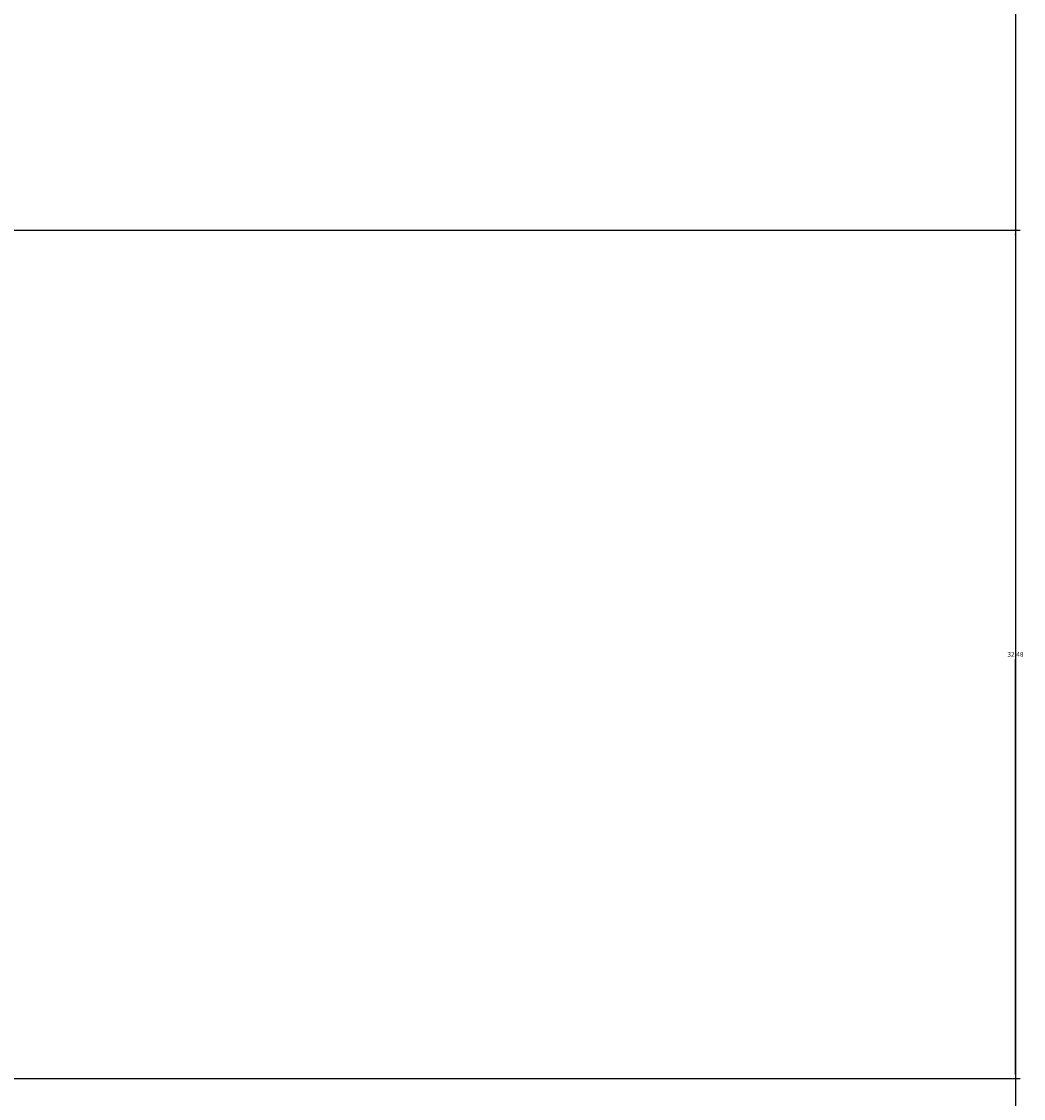
# Model space of a CAD drawing. Units: inches. Extents: x 1998 to 2588, y 1139 to 1977.
# Tile 121 of 134: x 2550 to 2588, y 1595 to 1637. Entities that reach past the tile are written whole.
import ezdxf

# ---------------------------------------------------------------- set-up
doc = ezdxf.new("R2010")
doc.units = ezdxf.units.IN
doc.layers.add('A-ANNO-DIMS', color=2, linetype='Continuous', lineweight=18)
doc.styles.get("Standard").update_dxf_attribs({"font": 'arial.ttf'})
doc.dimstyles.get("Standard").update_dxf_attribs({"dimtxt": 0.18, "dimasz": 0.18, "dimexe": 0.18, "dimexo": 0.0625, "dimgap": 0.09, "dimtad": 0, "dimtih": 1, "dimtoh": 1, "dimdec": 4, "dimzin": 0, "dimdsep": 46, "dimtxsty": 'Standard', "dimcen": 0.09, "dimadec": 0, "dimazin": 0, "dimtfac": 1, "dimtdec": 4, "dimtofl": 0, "dimtmove": 0, "dimatfit": 3, "dimfxl": 1, "dimtolj": 1, "dimtzin": 0, "dimarcsym": 0})

# ---------------------------------------------------------------- blocks, each defined once
blk = doc.blocks.new('*D24')
at = {"layer": 'A-ANNO-DIMS', "color": 0, "lineweight": -2, "transparency": 16777216}
for p, q in [((2398.535, 1911.232), (2588.309, 1911.232)), ((2588.129, 1911.052), (2588.129, 1570.164)), ((2588.129, 1228.912), (2588.129, 1569.8)), ((2527.535, 1228.732), (2588.309, 1228.732))]:
    blk.add_line(p, q, dxfattribs=at)
at = {"layer": 'A-ANNO-DIMS', "color": 0, "transparency": 16777216}
for points in [[(2588.099, 1911.052), (2588.159, 1911.052), (2588.129, 1911.232)], [(2588.099, 1228.912), (2588.159, 1228.912), (2588.129, 1228.732)]]:
    blk.add_solid(points, dxfattribs=at)
at = {"layer": 'Defpoints', "color": 0, "transparency": 16777216}
for p in [(2398.473, 1911.232), (2588.129, 1911.232), (2527.473, 1228.732)]:
    blk.add_point(p, dxfattribs=at)
at = {"layer": 'A-ANNO-DIMS', "color": 0, "transparency": 16777216, "insert": (2588.129, 1569.982), "char_height": 0.18, "attachment_point": 5}
blk.add_mtext('\\A1;682.5', dxfattribs=at)
blk = doc.blocks.new('*D39')
at = {"layer": 'A-ANNO-DIMS', "color": 0, "lineweight": -2, "transparency": 16777216}
for p, q in [((2115.035, 1628.742), (2588.309, 1628.742)), ((2588.129, 1628.562), (2588.129, 1612.685)), ((2588.129, 1596.444), (2588.129, 1612.321)), ((2115.035, 1596.264), (2588.309, 1596.264))]:
    blk.add_line(p, q, dxfattribs=at)
at = {"layer": 'A-ANNO-DIMS', "color": 0, "transparency": 16777216}
for points in [[(2588.099, 1628.562), (2588.159, 1628.562), (2588.129, 1628.742)], [(2588.099, 1596.444), (2588.159, 1596.444), (2588.129, 1596.264)]]:
    blk.add_solid(points, dxfattribs=at)
at = {"layer": 'Defpoints', "color": 0, "transparency": 16777216}
for p in [(2114.973, 1628.742), (2588.129, 1628.742), (2114.973, 1596.264)]:
    blk.add_point(p, dxfattribs=at)
at = {"layer": 'A-ANNO-DIMS', "color": 0, "transparency": 16777216, "insert": (2588.129, 1612.503), "char_height": 0.18, "attachment_point": 5}
blk.add_mtext('\\A1;32.48', dxfattribs=at)

msp = doc.modelspace()

# ---------------------------------------------------------------- dimensions: what is measured, and where the dimension line sits
at = {"layer": 'A-ANNO-DIMS'}
for base, p1, p2, override, picture, middle in [((2588.1286, 1911.2324), (2527.4729, 1228.7324), (2398.4729, 1911.2324), {"dimdec": 1, "dimlfac": 1, "dimrnd": 0, "dimzin": 0, "dimdsep": 46, "dimlunit": 2}, '*D24', (2588.1286, 1569.9824)), ((2588.1286, 1628.7416), (2114.9729, 1596.2642), (2114.9729, 1628.7416), {"dimdec": 2, "dimlfac": 1, "dimrnd": 0, "dimzin": 0, "dimdsep": 46, "dimlunit": 2}, '*D39', (2588.1286, 1612.5029))]:
    dim = msp.add_linear_dim(base=base, p1=p1, p2=p2, angle=90, dimstyle='Standard', override=override, dxfattribs=at)
    dim.commit()
    dim.dimension.update_dxf_attribs({"geometry": picture, "text_midpoint": middle})

doc.saveas('drawing.dxf')
